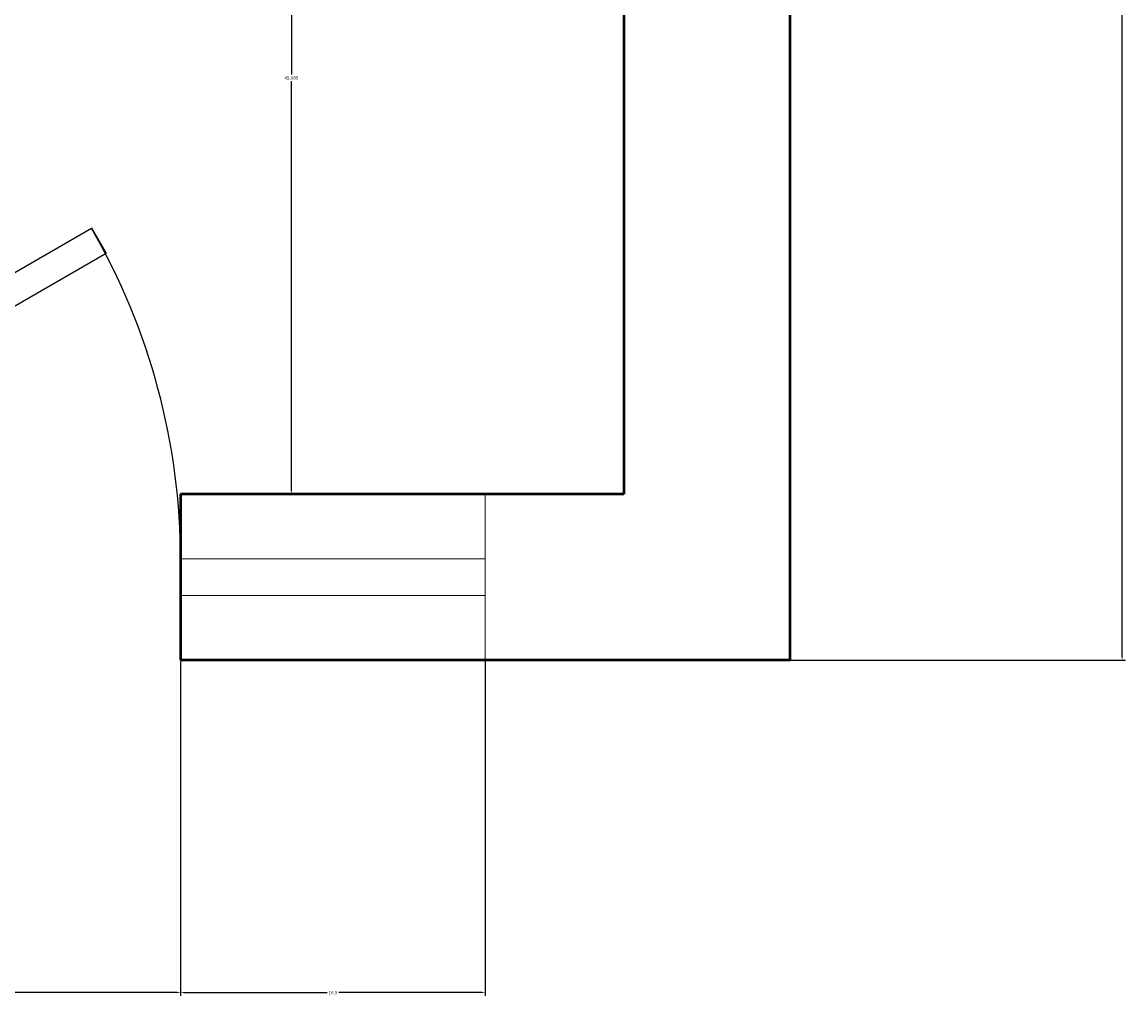
# Model space of a CAD drawing. Units: inches. Extents: x 2621 to 2849, y 2066 to 2463.
# Tile 4 of 28: x 2789 to 2849, y 2066 to 2119. Entities that reach past the tile are written whole.
import ezdxf

# ---------------------------------------------------------------- set-up
doc = ezdxf.new("R2010")
doc.units = ezdxf.units.IN
for name, color, linetype, lineweight in [('A-ANNO-DIMS', 2, 'Continuous', 18), ('A-DOOR', 3, 'Continuous', 25), ('A-GLAZ', 4, 'Continuous', 18), ('A-WALL', 7, 'Continuous', 50)]:
    doc.layers.add(name, color=color, linetype=linetype, lineweight=lineweight)
doc.styles.get("Standard").update_dxf_attribs({"font": 'arial.ttf'})
doc.dimstyles.get("Standard").update_dxf_attribs({"dimtxt": 0.18, "dimasz": 0.18, "dimexe": 0.18, "dimexo": 0.0625, "dimgap": 0.09, "dimtad": 0, "dimtih": 1, "dimtoh": 1, "dimdec": 4, "dimzin": 0, "dimdsep": 46, "dimtxsty": 'Standard', "dimcen": 0.09, "dimadec": 0, "dimazin": 0, "dimtfac": 1, "dimtdec": 4, "dimtofl": 0, "dimtmove": 0, "dimatfit": 3, "dimfxl": 1, "dimtolj": 1, "dimtzin": 0, "dimarcsym": 0})

# ---------------------------------------------------------------- blocks, each defined once
blk = doc.blocks.new('*U4')
for p, q in [((0, 0), (0, -6)), ((40, 0), (40, -6))]:
    blk.add_line(p, q)
blk.add_lwpolyline([(0, 0), (34.641, 20), (35.516, 18.484), (0.875, -1.516)], close=True)
blk.add_arc((0, 0), 40, 0, 30)
blk = doc.blocks.new('*D36')
at = {"layer": 'A-ANNO-DIMS', "color": 0, "lineweight": -2, "transparency": 16777216}
for p, q in [((2830.933, 2444.375), (2849.054, 2444.375)), ((2848.874, 2444.195), (2848.874, 2264.557)), ((2848.874, 2084.555), (2848.874, 2264.193)), ((2830.933, 2084.375), (2849.054, 2084.375))]:
    blk.add_line(p, q, dxfattribs=at)
at = {"layer": 'A-ANNO-DIMS', "color": 0, "transparency": 16777216}
for points in [[(2848.844, 2444.195), (2848.904, 2444.195), (2848.874, 2444.375)], [(2848.844, 2084.555), (2848.904, 2084.555), (2848.874, 2084.375)]]:
    blk.add_solid(points, dxfattribs=at)
at = {"layer": 'Defpoints', "color": 0, "transparency": 16777216}
for p in [(2830.87, 2444.375), (2848.874, 2444.375), (2830.87, 2084.375)]:
    blk.add_point(p, dxfattribs=at)
at = {"layer": 'A-ANNO-DIMS', "color": 0, "transparency": 16777216, "insert": (2848.874, 2264.375), "char_height": 0.18, "attachment_point": 5}
blk.add_mtext('\\A1;360', dxfattribs=at)
blk = doc.blocks.new('*D42')
at = {"layer": 'A-ANNO-DIMS', "color": 0, "lineweight": -2, "transparency": 16777216}
for p, q in [((2761.87, 2084.312), (2761.87, 2066.191)), ((2797.87, 2084.312), (2797.87, 2066.191)), ((2762.05, 2066.371), (2779.651, 2066.371)), ((2797.69, 2066.371), (2780.089, 2066.371))]:
    blk.add_line(p, q, dxfattribs=at)
at = {"layer": 'A-ANNO-DIMS', "color": 0, "transparency": 16777216}
for points in [[(2762.05, 2066.401), (2762.05, 2066.341), (2761.87, 2066.371)], [(2797.69, 2066.401), (2797.69, 2066.341), (2797.87, 2066.371)]]:
    blk.add_solid(points, dxfattribs=at)
at = {"layer": 'Defpoints', "color": 0, "transparency": 16777216}
for p in [(2761.87, 2084.375), (2797.87, 2084.375), (2797.87, 2066.371)]:
    blk.add_point(p, dxfattribs=at)
at = {"layer": 'A-ANNO-DIMS', "color": 0, "transparency": 16777216, "insert": (2779.87, 2066.371), "char_height": 0.18, "attachment_point": 5}
blk.add_mtext('\\A1;36', dxfattribs=at)
blk = doc.blocks.new('*D43')
at = {"layer": 'A-ANNO-DIMS', "color": 0, "lineweight": -2, "transparency": 16777216}
for p, q in [((2797.87, 2084.312), (2797.87, 2066.191)), ((2814.37, 2084.312), (2814.37, 2066.191)), ((2798.05, 2066.371), (2805.804, 2066.371)), ((2814.19, 2066.371), (2806.436, 2066.371))]:
    blk.add_line(p, q, dxfattribs=at)
at = {"layer": 'A-ANNO-DIMS', "color": 0, "transparency": 16777216}
for points in [[(2798.05, 2066.401), (2798.05, 2066.341), (2797.87, 2066.371)], [(2814.19, 2066.401), (2814.19, 2066.341), (2814.37, 2066.371)]]:
    blk.add_solid(points, dxfattribs=at)
at = {"layer": 'Defpoints', "color": 0, "transparency": 16777216}
for p in [(2797.87, 2084.375), (2814.37, 2084.375), (2814.37, 2066.371)]:
    blk.add_point(p, dxfattribs=at)
at = {"layer": 'A-ANNO-DIMS', "color": 0, "transparency": 16777216, "insert": (2806.12, 2066.371), "char_height": 0.18, "attachment_point": 5}
blk.add_mtext('\\A1;16.5', dxfattribs=at)
blk = doc.blocks.new('*D60')
at = {"layer": 'A-ANNO-DIMS', "color": 0, "lineweight": -2, "transparency": 16777216}
for p, q in [((2821.808, 2138.46), (2803.687, 2138.46)), ((2803.867, 2138.28), (2803.867, 2116.099)), ((2803.867, 2093.555), (2803.867, 2115.735)), ((2821.808, 2093.375), (2803.687, 2093.375))]:
    blk.add_line(p, q, dxfattribs=at)
at = {"layer": 'A-ANNO-DIMS', "color": 0, "transparency": 16777216}
for points in [[(2803.837, 2138.28), (2803.897, 2138.28), (2803.867, 2138.46)], [(2803.837, 2093.555), (2803.897, 2093.555), (2803.867, 2093.375)]]:
    blk.add_solid(points, dxfattribs=at)
at = {"layer": 'Defpoints', "color": 0, "transparency": 16777216}
for p in [(2803.867, 2138.46), (2821.87, 2138.46), (2821.87, 2093.375)]:
    blk.add_point(p, dxfattribs=at)
at = {"layer": 'A-ANNO-DIMS', "color": 0, "transparency": 16777216, "insert": (2803.867, 2115.917), "char_height": 0.18, "attachment_point": 5}
blk.add_mtext('\\A1;45.085', dxfattribs=at)

msp = doc.modelspace()

# ---------------------------------------------------------------- linework, layer by layer
at = {"layer": 'A-GLAZ'}
for p, q in [((2797.8701, 2089.8746), (2814.3701, 2089.8746)), ((2797.8701, 2087.8746), (2814.3701, 2087.8746))]:
    msp.add_line(p, q, dxfattribs=at)
for points in [[(2797.8701, 2084.3746), (2797.8701, 2093.3746)], [(2814.3701, 2093.3746), (2814.3701, 2084.3746)]]:
    msp.add_lwpolyline(points, dxfattribs=at)
at = {"layer": 'A-WALL'}
for p, q in [((2821.8701, 2371.3746), (2821.8701, 2093.3746)), ((2821.8701, 2093.3746), (2797.8701, 2093.3746)), ((2797.8701, 2093.3746), (2797.8701, 2084.3746))]:
    msp.add_line(p, q, dxfattribs=at)
msp.add_lwpolyline([(2761.8701, 2084.3746), (2638.8701, 2084.3746), (2638.8701, 2444.3746), (2830.8701, 2444.3746), (2830.8701, 2084.3746), (2797.8701, 2084.3746)], dxfattribs=at)

# ---------------------------------------------------------------- block references
at = {"layer": 'A-DOOR', "xscale": 0.9, "yscale": 0.9, "zscale": 0.9}
msp.add_blockref('*U4', (2761.8701, 2089.7746), dxfattribs=at)

# ---------------------------------------------------------------- dimensions: what is measured, and where the dimension line sits
at = {"layer": 'A-ANNO-DIMS'}
for base, p1, p2, override, picture, middle in [((2848.8736, 2444.3746), (2830.8701, 2084.3746), (2830.8701, 2444.3746), {"dimdec": 0, "dimlfac": 1, "dimrnd": 0, "dimzin": 0, "dimdsep": 46, "dimlunit": 2}, '*D36', (2848.8736, 2264.3746)), ((2803.8666, 2138.4598), (2821.8701, 2093.3746), (2821.8701, 2138.4598), {"dimdec": 3, "dimlfac": 1, "dimrnd": 0, "dimzin": 0, "dimdsep": 46, "dimlunit": 2}, '*D60', (2803.8666, 2115.9172))]:
    dim = msp.add_linear_dim(base=base, p1=p1, p2=p2, angle=90, dimstyle='Standard', override=override, dxfattribs=at)
    dim.commit()
    dim.dimension.update_dxf_attribs({"geometry": picture, "text_midpoint": middle})
for base, p1, p2, override, picture, middle in [((2797.8701, 2066.3711), (2761.8701, 2084.3746), (2797.8701, 2084.3746), {"dimdec": 0, "dimlfac": 1, "dimrnd": 0, "dimzin": 0, "dimdsep": 46, "dimlunit": 2}, '*D42', (2779.8701, 2066.3711)), ((2814.3701, 2066.3711), (2797.8701, 2084.3746), (2814.3701, 2084.3746), {"dimdec": 1, "dimlfac": 1, "dimrnd": 0, "dimzin": 0, "dimdsep": 46, "dimlunit": 2}, '*D43', (2806.1201, 2066.3711))]:
    dim = msp.add_linear_dim(base=base, p1=p1, p2=p2, dimstyle='Standard', override=override, dxfattribs=at)
    dim.commit()
    dim.dimension.update_dxf_attribs({"geometry": picture, "text_midpoint": middle})

doc.saveas('drawing.dxf')
